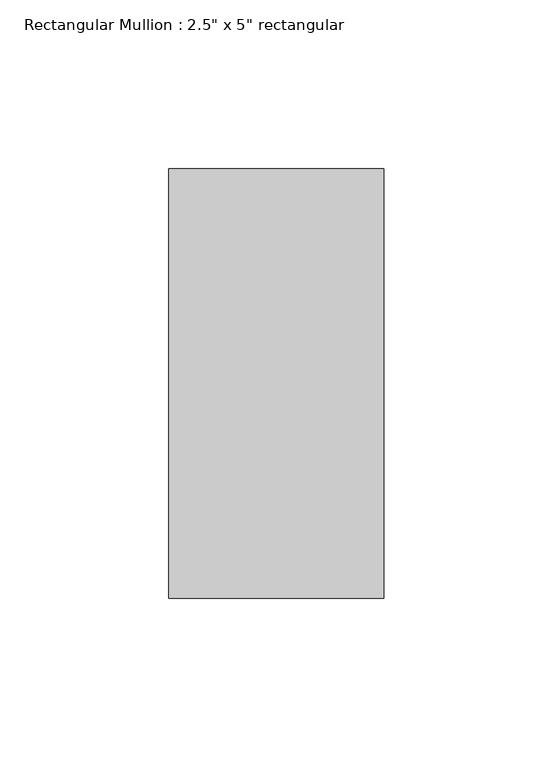
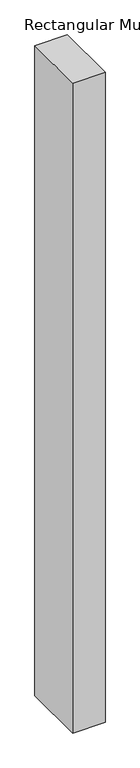
"""IFC4 building model written with IfcOpenShell, lengths in millimetres: member geometry."""

from ifc_helpers import new_model, si_unit, frame, origin, place, context, project, spatial, polyline, outline, extrude, source, transform, mapped, element, save


def member_97a07400(model_context):
    return source(origin(), model_context, "Body", "SweptSolid", [
        extrude(outline(polyline([(0.0, 63.5), (0.0, -63.5), (-63.5, -63.5), (-63.5, 63.5), (0.0, 63.5)])), frame((0.0, 0.0, -1339.8500001), z_axis=(0.0, 0.0, 1.0), x_axis=(1.0, 0.0, 0.0)), (0.0, 0.0, 1.0), 1339.8500001),
    ])


if __name__ == "__main__":
    model = new_model("IFC4")
    model_context = context("Model", 3, world=origin())
    ifc_project = project(units=[si_unit("LENGTHUNIT", "METRE", prefix="MILLI")], contexts=[model_context])
    site = spatial("IfcSite", under=ifc_project)
    building = spatial("IfcBuilding", under=site)
    placement = place(None, origin())
    member_shape = member_97a07400(model_context)
    element("IfcMember", 1, ObjectType="Rectangular Mullion : 2.5\" x 5\" rectangular", at=placement, inside=building, context=model_context, shape_type="MappedRepresentation", body=[
        mapped(member_shape, transform((0.0, 0.0, 0.0), x_axis=(1.0, 0.0, 0.0), y_axis=(0.0, 1.0, 0.0), z_axis=(0.0, 0.0, 1.0))),
    ])
    save(model, "model.ifc")

# Revit data of these elements
# Type "Rectangular Mullion : 2.5\" x 5\" rectangular"
#   built-in parameter 1007304 = 0.416667 (stored number, unit not read)
#   built-in parameter 1007301 = 0.104167 (stored number, unit not read)
#   built-in parameter 1007300 = 0.104167 (stored number, unit not read)
# Element 1 (IfcMember, "Rectangular Mullion : 2.5\" x 5\" rectangular")
#   Materials on its faces: "Aluminum"
# Materials
#   "Aluminum": class "Metal", colour RGB 247 247 247, transparency 0, Description = "Aluminum 6061", Cost = 0
